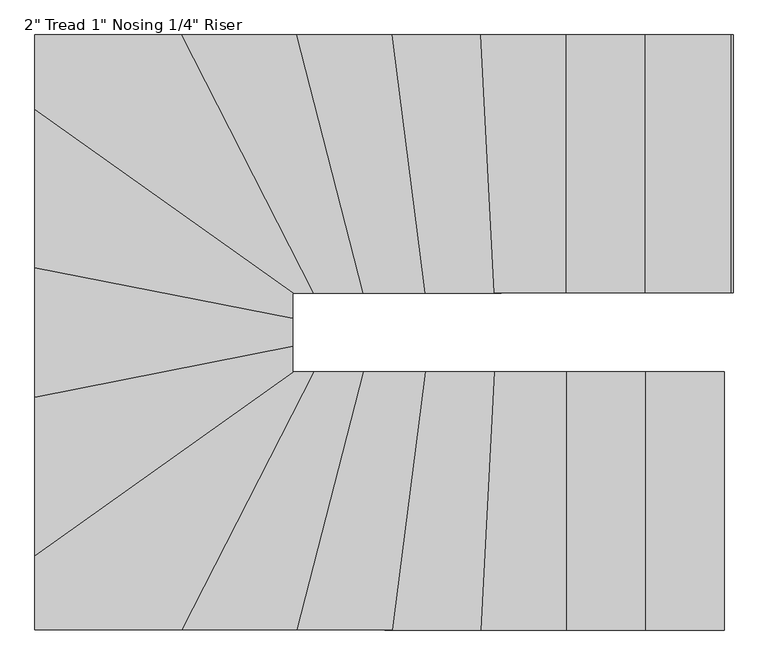
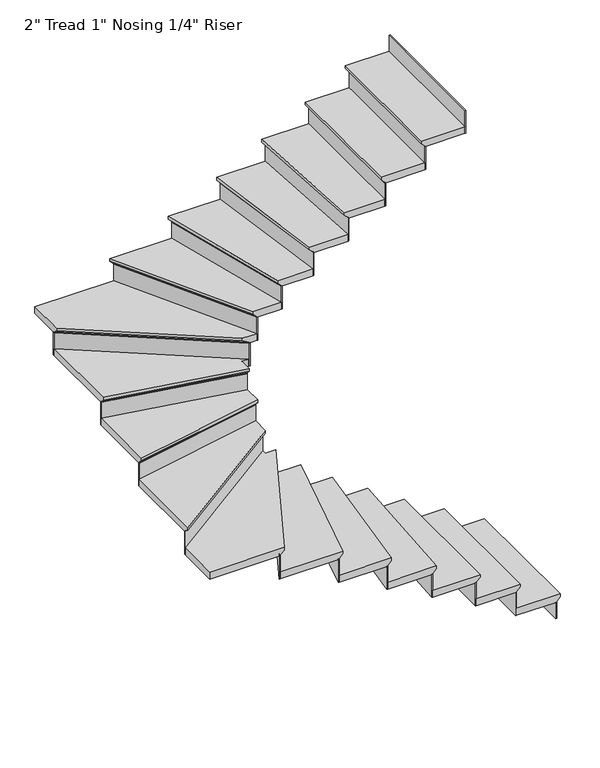
"""IFC4 building model written with IfcOpenShell, lengths in millimetres: stair flight geometry."""

from ifc_helpers import new_model, si_unit, origin, place, context, project, spatial, faceted_brep, source, transform, mapped, element, save


def stair_flight_2afbddc8(model_context):
    return source(origin(), model_context, "Body", "Brep", [
        faceted_brep([(-5773.8240284, 3285.2245992, 150.2833333), (-5773.8240284, 3285.2245992, 169.3333333), (-5773.8240284, 2370.8245992, 169.3333333), (-5773.8240284, 2370.8245992, 150.2833333), (-5799.2240284, 3285.2245992, 124.8833333), (-5799.2240284, 2370.8245992, 124.8833333), (-6078.6240284, 3285.2245992, 169.3333333), (-6078.6240284, 2370.8245992, 169.3333333), (-5799.2240284, 2370.8245992, 118.5333333), (-6078.6240284, 2370.8245992, 118.5333333), (-6078.6240284, 3285.2245992, 118.5333333), (-5799.2240284, 3285.2245992, 118.5333333)], [[[0, 1, 2, 3]], [[4, 0, 3, 5]], [[2, 1, 6, 7]], [[8, 9, 10, 11]], [[2, 7, 9, 8, 5, 3]], [[8, 11, 4, 5]], [[6, 1, 0, 4, 11, 10]], [[7, 6, 10, 9]]]),
        faceted_brep([(-5799.2240284, 3285.2245992, 118.5333333), (-5799.2240284, 3285.2245992, 0.0), (-5805.5740284, 3285.2245992, 0.0), (-5805.5740284, 3285.2245992, 118.5333333), (-5799.2240284, 2370.8245992, 118.5333333), (-5805.5740284, 2370.8245992, 118.5333333), (-5805.5740284, 2370.8245992, 0.0), (-5799.2240284, 2370.8245992, 0.0)], [[[0, 1, 2, 3]], [[4, 5, 6, 7]], [[1, 0, 4, 7]], [[2, 1, 7, 6]], [[3, 2, 6, 5]], [[0, 3, 5, 4]]]),
        faceted_brep([(-6078.6240284, 3285.2245992, 287.8666667), (-6078.6240284, 3285.2245992, 118.5333333), (-6084.9740284, 3285.2245992, 118.5333333), (-6084.9740284, 3285.2245992, 287.8666667), (-6078.6240284, 2370.8245992, 287.8666667), (-6084.9740284, 2370.8245992, 287.8666667), (-6084.9740284, 2370.8245992, 118.5333333), (-6078.6240284, 2370.8245992, 118.5333333)], [[[0, 1, 2, 3]], [[4, 5, 6, 7]], [[1, 0, 4, 7]], [[2, 1, 7, 6]], [[3, 2, 6, 5]], [[0, 3, 5, 4]]]),
        faceted_brep([(-6053.2240284, 2370.8245992, 338.6666667), (-6053.2240284, 3285.2245992, 338.6666667), (-6358.0240284, 3285.2245992, 338.6666667), (-6358.0240284, 2370.8245992, 338.6666667), (-6078.6240284, 2370.8245992, 287.8666667), (-6358.0240284, 2370.8245992, 287.8666667), (-6358.0240284, 3285.2245992, 287.8666667), (-6078.6240284, 3285.2245992, 287.8666667), (-6078.6240284, 2370.8245992, 294.2166667), (-6053.2240284, 2370.8245992, 319.6166667), (-6078.6240284, 3285.2245992, 294.2166667), (-6053.2240284, 3285.2245992, 319.6166667)], [[[0, 1, 2, 3]], [[4, 5, 6, 7]], [[0, 3, 5, 4, 8, 9]], [[4, 7, 10, 8]], [[2, 1, 11, 10, 7, 6]], [[3, 2, 6, 5]], [[11, 1, 0, 9]], [[10, 11, 9, 8]]]),
        faceted_brep([(-6358.0240284, 3285.2245992, 457.2), (-6358.0240284, 3285.2245992, 287.8666667), (-6364.3740284, 3285.2245992, 287.8666667), (-6364.3740284, 3285.2245992, 457.2), (-6358.0240284, 2370.8245992, 457.2), (-6364.3740284, 2370.8245992, 457.2), (-6364.3740284, 2370.8245992, 287.8666667), (-6358.0240284, 2370.8245992, 287.8666667)], [[[0, 1, 2, 3]], [[4, 5, 6, 7]], [[1, 0, 4, 7]], [[2, 1, 7, 6]], [[3, 2, 6, 5]], [[0, 3, 5, 4]]]),
        faceted_brep([(-6332.6240284, 2370.8245992, 508.0), (-6332.6240284, 3285.2245992, 508.0), (-6613.6911898, 3285.2245992, 508.0), (-6661.2254602, 2370.8245992, 508.0), (-6358.0240284, 2370.8245992, 457.2), (-6661.2254602, 2370.8245992, 457.2), (-6613.6911898, 3285.2245992, 457.2), (-6358.0240284, 3285.2245992, 457.2), (-6358.0240284, 2370.8245992, 463.55), (-6332.6240284, 2370.8245992, 488.95), (-6358.0240284, 3285.2245992, 463.55), (-6332.6240284, 3285.2245992, 488.95)], [[[0, 1, 2, 3]], [[4, 5, 6, 7]], [[0, 3, 5, 4, 8, 9]], [[4, 7, 10, 8]], [[2, 1, 11, 10, 7, 6]], [[3, 2, 6, 5]], [[11, 1, 0, 9]], [[10, 11, 9, 8]]]),
        faceted_brep([(-6613.6911898, 3285.2245992, 626.5333333), (-6613.6911898, 3285.2245992, 457.2), (-6620.049764, 3285.2245992, 457.2), (-6620.049764, 3285.2245992, 626.5333333), (-6661.2254602, 2370.8245992, 626.5333333), (-6667.5840344, 2370.8245992, 626.5333333), (-6667.5840344, 2370.8245992, 457.2), (-6661.2254602, 2370.8245992, 457.2)], [[[0, 1, 2, 3]], [[4, 5, 6, 7]], [[1, 0, 4, 7]], [[2, 1, 7, 6]], [[3, 2, 6, 5]], [[0, 3, 5, 4]]]),
        faceted_brep([(-6635.7911636, 2370.8245992, 677.3333333), (-6588.2568932, 3285.2245992, 677.3333333), (-6857.8578897, 3285.2245992, 677.3333333), (-6976.2139413, 2370.8245992, 677.3333333), (-6661.2254602, 2370.8245992, 626.5333333), (-6976.2139413, 2370.8245992, 626.5333333), (-6857.8578897, 3285.2245992, 626.5333333), (-6613.6911898, 3285.2245992, 626.5333333), (-6661.2254602, 2370.8245992, 632.8833333), (-6635.7911636, 2370.8245992, 658.2833333), (-6613.6911898, 3285.2245992, 632.8833333), (-6588.2568932, 3285.2245992, 658.2833333)], [[[0, 1, 2, 3]], [[4, 5, 6, 7]], [[0, 3, 5, 4, 8, 9]], [[4, 7, 10, 8]], [[2, 1, 11, 10, 7, 6]], [[3, 2, 6, 5]], [[11, 1, 0, 9]], [[10, 11, 9, 8]]]),
        faceted_brep([(-6857.8578897, 3285.2245992, 795.8666667), (-6857.8578897, 3285.2245992, 626.5333333), (-6864.2608614, 3285.2245992, 626.5333333), (-6864.2608614, 3285.2245992, 795.8666667), (-6976.2139413, 2370.8245992, 795.8666667), (-6982.6169131, 2370.8245992, 795.8666667), (-6982.6169131, 2370.8245992, 626.5333333), (-6976.2139413, 2370.8245992, 626.5333333)], [[[0, 1, 2, 3]], [[4, 5, 6, 7]], [[1, 0, 4, 7]], [[2, 1, 7, 6]], [[3, 2, 6, 5]], [[0, 3, 5, 4]]]),
        faceted_brep([(-6950.6020542, 2370.8245992, 846.6666667), (-6832.2460026, 3285.2245992, 846.6666667), (-7079.4851121, 3285.2245992, 846.6666667), (-7314.6155595, 2370.8245992, 846.6666667), (-6976.2139413, 2370.8245992, 795.8666667), (-7314.6155595, 2370.8245992, 795.8666667), (-7079.4851121, 3285.2245992, 795.8666667), (-6857.8578897, 3285.2245992, 795.8666667), (-6976.2139413, 2370.8245992, 802.2166667), (-6950.6020542, 2370.8245992, 827.6166667), (-6857.8578897, 3285.2245992, 802.2166667), (-6832.2460026, 3285.2245992, 827.6166667)], [[[0, 1, 2, 3]], [[4, 5, 6, 7]], [[0, 3, 5, 4, 8, 9]], [[4, 7, 10, 8]], [[2, 1, 11, 10, 7, 6]], [[3, 2, 6, 5]], [[11, 1, 0, 9]], [[10, 11, 9, 8]]]),
        faceted_brep([(-7079.4851121, 3285.2245992, 965.2), (-7079.4851121, 3285.2245992, 795.8666667), (-7086.041689, 3285.2245992, 795.8666667), (-7086.041689, 3285.2245992, 965.2), (-7314.6155595, 2370.8245992, 965.2), (-7321.1721364, 2370.8245992, 965.2), (-7321.1721364, 2370.8245992, 795.8666667), (-7314.6155595, 2370.8245992, 795.8666667)], [[[0, 1, 2, 3]], [[4, 5, 6, 7]], [[1, 0, 4, 7]], [[2, 1, 7, 6]], [[3, 2, 6, 5]], [[0, 3, 5, 4]]]),
        faceted_brep([(-7288.3892521, 2370.8245992, 1016.0), (-7053.2588047, 3285.2245992, 1016.0), (-7255.8317482, 3285.2245992, 1016.0), (-7724.6563696, 2370.8245992, 1016.0), (-7314.6155595, 2370.8245992, 965.2), (-7724.6563696, 2370.8245992, 965.2), (-7255.8317482, 3285.2245992, 965.2), (-7079.4851121, 3285.2245992, 965.2), (-7314.6155595, 2370.8245992, 971.55), (-7288.3892521, 2370.8245992, 996.95), (-7079.4851121, 3285.2245992, 971.55), (-7053.2588047, 3285.2245992, 996.95)], [[[0, 1, 2, 3]], [[4, 5, 6, 7]], [[0, 3, 5, 4, 8, 9]], [[4, 7, 10, 8]], [[2, 1, 11, 10, 7, 6]], [[3, 2, 6, 5]], [[11, 1, 0, 9]], [[10, 11, 9, 8]]]),
        faceted_brep([(-7255.8317482, 3285.2245992, 1134.5333333), (-7255.8317482, 3285.2245992, 965.2), (-7262.9677314, 3285.2245992, 965.2), (-7262.9677314, 3285.2245992, 1134.5333333), (-7724.6563696, 2370.8245992, 1134.5333333), (-7731.7923527, 2370.8245992, 1134.5333333), (-7731.7923527, 2370.8245992, 965.2), (-7724.6563696, 2370.8245992, 965.2)], [[[0, 1, 2, 3]], [[4, 5, 6, 7]], [[1, 0, 4, 7]], [[2, 1, 7, 6]], [[3, 2, 6, 5]], [[0, 3, 5, 4]]]),
        faceted_brep([(-8215.9557202, 2664.5057329, 1185.3333333), (-8215.9557202, 2370.8245992, 1185.3333333), (-7696.112437, 2370.8245992, 1185.3333333), (-7227.2878157, 3285.2245992, 1185.3333333), (-7301.5557202, 3285.2245992, 1185.3333333), (-7301.5557202, 3314.7796821, 1185.3333333), (-8215.9557202, 2370.8245992, 1134.5333333), (-8215.9557202, 2664.5057329, 1134.5333333), (-7301.5557202, 3314.7796821, 1134.5333333), (-7301.5557202, 3285.2245992, 1134.5333333), (-7255.8317482, 3285.2245992, 1134.5333333), (-7724.6563696, 2370.8245992, 1134.5333333), (-7724.6563696, 2370.8245992, 1140.8833333), (-7696.112437, 2370.8245992, 1166.2833333), (-7255.8317482, 3285.2245992, 1140.8833333), (-7227.2878157, 3285.2245992, 1166.2833333)], [[[0, 1, 2, 3, 4, 5]], [[6, 7, 8, 9, 10, 11]], [[1, 0, 7, 6]], [[2, 1, 6, 11, 12, 13]], [[11, 10, 14, 12]], [[4, 3, 15, 14, 10, 9]], [[5, 4, 9, 8]], [[0, 5, 8, 7]], [[15, 3, 2, 13]], [[14, 15, 13, 12]]]),
        faceted_brep([(-7301.5557202, 3314.7796821, 1303.8666667), (-7301.5557202, 3314.7796821, 1134.5333333), (-7301.5557202, 3322.5716569, 1134.5333333), (-7301.5557202, 3322.5716569, 1303.8666667), (-8215.9557202, 2664.5057329, 1303.8666667), (-8215.9557202, 2672.2977077, 1303.8666667), (-8215.9557202, 2672.2977077, 1134.5333333), (-8215.9557202, 2664.5057329, 1134.5333333)], [[[0, 1, 2, 3]], [[4, 5, 6, 7]], [[1, 0, 4, 7]], [[2, 1, 7, 6]], [[3, 2, 6, 5]], [[0, 3, 5, 4]]]),
        faceted_brep([(-8215.9557202, 2633.3378337, 1354.6666667), (-7301.5557202, 3283.6117829, 1354.6666667), (-7301.5557202, 3401.2337691, 1354.6666667), (-8215.9557202, 3220.9929128, 1354.6666667), (-8215.9557202, 2664.5057329, 1303.8666667), (-8215.9557202, 3220.9929128, 1303.8666667), (-7301.5557202, 3401.2337691, 1303.8666667), (-7301.5557202, 3314.7796821, 1303.8666667), (-8215.9557202, 2664.5057329, 1310.2166667), (-8215.9557202, 2633.3378337, 1335.6166667), (-7301.5557202, 3314.7796821, 1310.2166667), (-7301.5557202, 3283.6117829, 1335.6166667)], [[[0, 1, 2, 3]], [[4, 5, 6, 7]], [[0, 3, 5, 4, 8, 9]], [[4, 7, 10, 8]], [[2, 1, 11, 10, 7, 6]], [[3, 2, 6, 5]], [[11, 1, 0, 9]], [[10, 11, 9, 8]]]),
        faceted_brep([(-7301.5557202, 3401.2337691, 1473.2), (-7301.5557202, 3401.2337691, 1303.8666667), (-7301.5557202, 3407.7059546, 1303.8666667), (-7301.5557202, 3407.7059546, 1473.2), (-8215.9557202, 3220.9929128, 1473.2), (-8215.9557202, 3227.4650983, 1473.2), (-8215.9557202, 3227.4650983, 1303.8666667), (-8215.9557202, 3220.9929128, 1303.8666667)], [[[0, 1, 2, 3]], [[4, 5, 6, 7]], [[1, 0, 4, 7]], [[2, 1, 7, 6]], [[3, 2, 6, 5]], [[0, 3, 5, 4]]]),
        faceted_brep([(-8215.9557202, 3195.1041711, 1524.0), (-7301.5557202, 3375.3450274, 1524.0), (-7301.5557202, 3500.3929128, 1524.0), (-8215.9557202, 3680.6337691, 1524.0), (-8215.9557202, 3220.9929128, 1473.2), (-8215.9557202, 3680.6337691, 1473.2), (-7301.5557202, 3500.3929128, 1473.2), (-7301.5557202, 3401.2337691, 1473.2), (-8215.9557202, 3220.9929128, 1479.55), (-8215.9557202, 3195.1041711, 1504.95), (-7301.5557202, 3401.2337691, 1479.55), (-7301.5557202, 3375.3450274, 1504.95)], [[[0, 1, 2, 3]], [[4, 5, 6, 7]], [[0, 3, 5, 4, 8, 9]], [[4, 7, 10, 8]], [[2, 1, 11, 10, 7, 6]], [[3, 2, 6, 5]], [[11, 1, 0, 9]], [[10, 11, 9, 8]]]),
        faceted_brep([(-7301.5557202, 3500.3929128, 1642.5333333), (-7301.5557202, 3500.3929128, 1473.2), (-7301.5557202, 3506.8650983, 1473.2), (-7301.5557202, 3506.8650983, 1642.5333333), (-8215.9557202, 3680.6337691, 1642.5333333), (-8215.9557202, 3687.1059546, 1642.5333333), (-8215.9557202, 3687.1059546, 1473.2), (-8215.9557202, 3680.6337691, 1473.2)], [[[0, 1, 2, 3]], [[4, 5, 6, 7]], [[1, 0, 4, 7]], [[2, 1, 7, 6]], [[3, 2, 6, 5]], [[0, 3, 5, 4]]]),
        faceted_brep([(-8215.9557202, 3654.7450274, 1693.3333333), (-7301.5557202, 3474.5041711, 1693.3333333), (-7301.5557202, 3564.6245992, 1693.3333333), (-7255.4602457, 3564.6245992, 1693.3333333), (-8215.9557202, 4247.6792639, 1693.3333333), (-8215.9557202, 3680.6337691, 1642.5333333), (-8215.9557202, 4247.6792639, 1642.5333333), (-7255.4602457, 3564.6245992, 1642.5333333), (-7301.5557202, 3564.6245992, 1642.5333333), (-7301.5557202, 3500.3929128, 1642.5333333), (-8215.9557202, 3680.6337691, 1648.8833333), (-8215.9557202, 3654.7450274, 1674.2833333), (-7301.5557202, 3500.3929128, 1648.8833333), (-7301.5557202, 3474.5041711, 1674.2833333)], [[[0, 1, 2, 3, 4]], [[5, 6, 7, 8, 9]], [[0, 4, 6, 5, 10, 11]], [[5, 9, 12, 10]], [[2, 1, 13, 12, 9, 8]], [[3, 2, 8, 7]], [[4, 3, 7, 6]], [[13, 1, 0, 11]], [[12, 13, 11, 10]]]),
        faceted_brep([(-7255.4602457, 3564.6245992, 1811.8666667), (-7255.4602457, 3564.6245992, 1642.5333333), (-7244.5033532, 3564.6245992, 1642.5333333), (-7244.5033532, 3564.6245992, 1811.8666667), (-8215.9557202, 4247.6792639, 1811.8666667), (-8215.9557202, 4255.4712387, 1811.8666667), (-8215.9557202, 4255.4712387, 1642.5333333), (-8215.9557202, 4247.6792639, 1642.5333333)], [[[0, 1, 2, 3]], [[4, 5, 6, 7]], [[1, 0, 4, 7]], [[2, 1, 7, 6]], [[3, 2, 6, 5]], [[0, 3, 5, 4]]]),
        faceted_brep([(-7667.5685045, 4479.0245992, 1862.6666667), (-8215.9557202, 4479.0245992, 1862.6666667), (-8215.9557202, 4216.5113647, 1862.6666667), (-7299.2878157, 3564.6245992, 1862.6666667), (-7198.7438832, 3564.6245992, 1862.6666667), (-8215.9557202, 4479.0245992, 1811.8666667), (-7667.5685045, 4479.0245992, 1811.8666667), (-7198.7438832, 3564.6245992, 1811.8666667), (-7255.4602457, 3564.6245992, 1811.8666667), (-8215.9557202, 4247.6792639, 1811.8666667), (-8215.9557202, 4247.6792639, 1818.2166667), (-8215.9557202, 4216.5113647, 1843.6166667), (-7255.4602457, 3564.6245992, 1818.2166667), (-7299.2878157, 3564.6245992, 1843.6166667)], [[[0, 1, 2, 3, 4]], [[5, 6, 7, 8, 9]], [[1, 0, 6, 5]], [[2, 1, 5, 9, 10, 11]], [[9, 8, 12, 10]], [[4, 3, 13, 12, 8, 7]], [[0, 4, 7, 6]], [[13, 3, 2, 11]], [[12, 13, 11, 10]]]),
        faceted_brep([(-7198.7438832, 3564.6245992, 1981.2), (-7198.7438832, 3564.6245992, 1811.8666667), (-7191.6079, 3564.6245992, 1811.8666667), (-7191.6079, 3564.6245992, 1981.2), (-7667.5685045, 4479.0245992, 1981.2), (-7660.4325213, 4479.0245992, 1981.2), (-7660.4325213, 4479.0245992, 1811.8666667), (-7667.5685045, 4479.0245992, 1811.8666667)], [[[0, 1, 2, 3]], [[4, 5, 6, 7]], [[1, 0, 4, 7]], [[2, 1, 7, 6]], [[3, 2, 6, 5]], [[0, 3, 5, 4]]]),
        faceted_brep([(-7696.112437, 4479.0245992, 2032.0), (-7227.2878157, 3564.6245992, 2032.0), (-7027.0324972, 3564.6245992, 2032.0), (-7262.1629446, 4479.0245992, 2032.0), (-7667.5685045, 4479.0245992, 1981.2), (-7262.1629446, 4479.0245992, 1981.2), (-7027.0324972, 3564.6245992, 1981.2), (-7198.7438832, 3564.6245992, 1981.2), (-7667.5685045, 4479.0245992, 1987.55), (-7696.112437, 4479.0245992, 2012.95), (-7198.7438832, 3564.6245992, 1987.55), (-7227.2878157, 3564.6245992, 2012.95)], [[[0, 1, 2, 3]], [[4, 5, 6, 7]], [[0, 3, 5, 4, 8, 9]], [[4, 7, 10, 8]], [[2, 1, 11, 10, 7, 6]], [[3, 2, 6, 5]], [[11, 1, 0, 9]], [[10, 11, 9, 8]]]),
        faceted_brep([(-7027.0324972, 3564.6245992, 2150.5333333), (-7027.0324972, 3564.6245992, 1981.2), (-7020.4759203, 3564.6245992, 1981.2), (-7020.4759203, 3564.6245992, 2150.5333333), (-7262.1629446, 4479.0245992, 2150.5333333), (-7255.6063678, 4479.0245992, 2150.5333333), (-7255.6063678, 4479.0245992, 1981.2), (-7262.1629446, 4479.0245992, 1981.2)], [[[0, 1, 2, 3]], [[4, 5, 6, 7]], [[1, 0, 4, 7]], [[2, 1, 7, 6]], [[3, 2, 6, 5]], [[0, 3, 5, 4]]]),
        faceted_brep([(-7288.3892521, 4479.0245992, 2201.3333333), (-7053.2588047, 3564.6245992, 2201.3333333), (-6806.6341154, 3564.6245992, 2201.3333333), (-6924.9901671, 4479.0245992, 2201.3333333), (-7262.1629446, 4479.0245992, 2150.5333333), (-6924.9901671, 4479.0245992, 2150.5333333), (-6806.6341154, 3564.6245992, 2150.5333333), (-7027.0324972, 3564.6245992, 2150.5333333), (-7262.1629446, 4479.0245992, 2156.8833333), (-7288.3892521, 4479.0245992, 2182.2833333), (-7027.0324972, 3564.6245992, 2156.8833333), (-7053.2588047, 3564.6245992, 2182.2833333)], [[[0, 1, 2, 3]], [[4, 5, 6, 7]], [[0, 3, 5, 4, 8, 9]], [[4, 7, 10, 8]], [[2, 1, 11, 10, 7, 6]], [[3, 2, 6, 5]], [[11, 1, 0, 9]], [[10, 11, 9, 8]]]),
        faceted_brep([(-6806.6341154, 3564.6245992, 2319.8666667), (-6806.6341154, 3564.6245992, 2150.5333333), (-6800.2311437, 3564.6245992, 2150.5333333), (-6800.2311437, 3564.6245992, 2319.8666667), (-6924.9901671, 4479.0245992, 2319.8666667), (-6918.5871953, 4479.0245992, 2319.8666667), (-6918.5871953, 4479.0245992, 2150.5333333), (-6924.9901671, 4479.0245992, 2150.5333333)], [[[0, 1, 2, 3]], [[4, 5, 6, 7]], [[1, 0, 4, 7]], [[2, 1, 7, 6]], [[3, 2, 6, 5]], [[0, 3, 5, 4]]]),
        faceted_brep([(-6950.6020542, 4479.0245992, 2370.6666667), (-6832.2460026, 3564.6245992, 2370.6666667), (-6562.8225965, 3564.6245992, 2370.6666667), (-6610.3568669, 4479.0245992, 2370.6666667), (-6924.9901671, 4479.0245992, 2319.8666667), (-6610.3568669, 4479.0245992, 2319.8666667), (-6562.8225965, 3564.6245992, 2319.8666667), (-6806.6341154, 3564.6245992, 2319.8666667), (-6924.9901671, 4479.0245992, 2326.2166667), (-6950.6020542, 4479.0245992, 2351.6166667), (-6806.6341154, 3564.6245992, 2326.2166667), (-6832.2460026, 3564.6245992, 2351.6166667)], [[[0, 1, 2, 3]], [[4, 5, 6, 7]], [[0, 3, 5, 4, 8, 9]], [[4, 7, 10, 8]], [[2, 1, 11, 10, 7, 6]], [[3, 2, 6, 5]], [[11, 1, 0, 9]], [[10, 11, 9, 8]]]),
        faceted_brep([(-6562.8225965, 3564.6245992, 2489.2), (-6562.8225965, 3564.6245992, 2319.8666667), (-6556.4640223, 3564.6245992, 2319.8666667), (-6556.4640223, 3564.6245992, 2489.2), (-6610.3568669, 4479.0245992, 2489.2), (-6603.9982928, 4479.0245992, 2489.2), (-6603.9982928, 4479.0245992, 2319.8666667), (-6610.3568669, 4479.0245992, 2319.8666667)], [[[0, 1, 2, 3]], [[4, 5, 6, 7]], [[1, 0, 4, 7]], [[2, 1, 7, 6]], [[3, 2, 6, 5]], [[0, 3, 5, 4]]]),
        faceted_brep([(-6635.7911636, 4479.0245992, 2540.0), (-6588.2568932, 3564.6245992, 2540.0), (-6307.2240284, 3564.6245992, 2540.0), (-6307.2240284, 4479.0245992, 2540.0), (-6610.3568669, 4479.0245992, 2489.2), (-6307.2240284, 4479.0245992, 2489.2), (-6307.2240284, 3564.6245992, 2489.2), (-6562.8225965, 3564.6245992, 2489.2), (-6610.3568669, 4479.0245992, 2495.55), (-6635.7911636, 4479.0245992, 2520.95), (-6562.8225965, 3564.6245992, 2495.55), (-6588.2568932, 3564.6245992, 2520.95)], [[[0, 1, 2, 3]], [[4, 5, 6, 7]], [[0, 3, 5, 4, 8, 9]], [[4, 7, 10, 8]], [[2, 1, 11, 10, 7, 6]], [[3, 2, 6, 5]], [[11, 1, 0, 9]], [[10, 11, 9, 8]]]),
        faceted_brep([(-6307.2240284, 3564.6245992, 2658.5333333), (-6307.2240284, 3564.6245992, 2489.2), (-6300.8740284, 3564.6245992, 2489.2), (-6300.8740284, 3564.6245992, 2658.5333333), (-6307.2240284, 4479.0245992, 2658.5333333), (-6300.8740284, 4479.0245992, 2658.5333333), (-6300.8740284, 4479.0245992, 2489.2), (-6307.2240284, 4479.0245992, 2489.2)], [[[0, 1, 2, 3]], [[4, 5, 6, 7]], [[1, 0, 4, 7]], [[2, 1, 7, 6]], [[3, 2, 6, 5]], [[0, 3, 5, 4]]]),
        faceted_brep([(-6332.6240284, 4479.0245992, 2709.3333333), (-6332.6240284, 3564.6245992, 2709.3333333), (-6027.8240284, 3564.6245992, 2709.3333333), (-6027.8240284, 4479.0245992, 2709.3333333), (-6307.2240284, 4479.0245992, 2658.5333333), (-6027.8240284, 4479.0245992, 2658.5333333), (-6027.8240284, 3564.6245992, 2658.5333333), (-6307.2240284, 3564.6245992, 2658.5333333), (-6307.2240284, 4479.0245992, 2664.8833333), (-6332.6240284, 4479.0245992, 2690.2833333), (-6307.2240284, 3564.6245992, 2664.8833333), (-6332.6240284, 3564.6245992, 2690.2833333)], [[[0, 1, 2, 3]], [[4, 5, 6, 7]], [[0, 3, 5, 4, 8, 9]], [[4, 7, 10, 8]], [[2, 1, 11, 10, 7, 6]], [[3, 2, 6, 5]], [[11, 1, 0, 9]], [[10, 11, 9, 8]]]),
        faceted_brep([(-6027.8240284, 3564.6245992, 2827.8666667), (-6027.8240284, 3564.6245992, 2658.5333333), (-6021.4740284, 3564.6245992, 2658.5333333), (-6021.4740284, 3564.6245992, 2827.8666667), (-6027.8240284, 4479.0245992, 2827.8666667), (-6021.4740284, 4479.0245992, 2827.8666667), (-6021.4740284, 4479.0245992, 2658.5333333), (-6027.8240284, 4479.0245992, 2658.5333333)], [[[0, 1, 2, 3]], [[4, 5, 6, 7]], [[1, 0, 4, 7]], [[2, 1, 7, 6]], [[3, 2, 6, 5]], [[0, 3, 5, 4]]]),
        faceted_brep([(-5748.4240284, 3564.6245992, 2997.2), (-5748.4240284, 3564.6245992, 2827.8666667), (-5742.0740284, 3564.6245992, 2827.8666667), (-5742.0740284, 3564.6245992, 2997.2), (-5748.4240284, 4479.0245992, 2997.2), (-5742.0740284, 4479.0245992, 2997.2), (-5742.0740284, 4479.0245992, 2827.8666667), (-5748.4240284, 4479.0245992, 2827.8666667)], [[[0, 1, 2, 3]], [[4, 5, 6, 7]], [[1, 0, 4, 7]], [[2, 1, 7, 6]], [[3, 2, 6, 5]], [[0, 3, 5, 4]]]),
        faceted_brep([(-6053.2240284, 4479.0245992, 2878.6666667), (-6053.2240284, 3564.6245992, 2878.6666667), (-5748.4240284, 3564.6245992, 2878.6666667), (-5748.4240284, 4479.0245992, 2878.6666667), (-6027.8240284, 4479.0245992, 2827.8666667), (-5748.4240284, 4479.0245992, 2827.8666667), (-5748.4240284, 3564.6245992, 2827.8666667), (-6027.8240284, 3564.6245992, 2827.8666667), (-6027.8240284, 4479.0245992, 2834.2166667), (-6053.2240284, 4479.0245992, 2859.6166667), (-6027.8240284, 3564.6245992, 2834.2166667), (-6053.2240284, 3564.6245992, 2859.6166667)], [[[0, 1, 2, 3]], [[4, 5, 6, 7]], [[0, 3, 5, 4, 8, 9]], [[4, 7, 10, 8]], [[2, 1, 11, 10, 7, 6]], [[3, 2, 6, 5]], [[11, 1, 0, 9]], [[10, 11, 9, 8]]]),
    ])


if __name__ == "__main__":
    model = new_model("IFC4")
    model_context = context("Model", 3, world=origin())
    ifc_project = project(units=[si_unit("LENGTHUNIT", "METRE", prefix="MILLI")], contexts=[model_context])
    site = spatial("IfcSite", under=ifc_project)
    building = spatial("IfcBuilding", under=site)
    placement = place(None, origin())
    stair_flight_shape = stair_flight_2afbddc8(model_context)
    element("IfcStairFlight", 1, ObjectType="2\" Tread 1\" Nosing 1/4\" Riser", at=placement, inside=building, context=model_context, shape_type="MappedRepresentation", body=[
        mapped(stair_flight_shape, transform((0.0, 0.0, 0.0), x_axis=(1.0, 0.0, 0.0), y_axis=(0.0, 1.0, 0.0), z_axis=(0.0, 0.0, 1.0))),
    ])
    save(model, "model.ifc")
